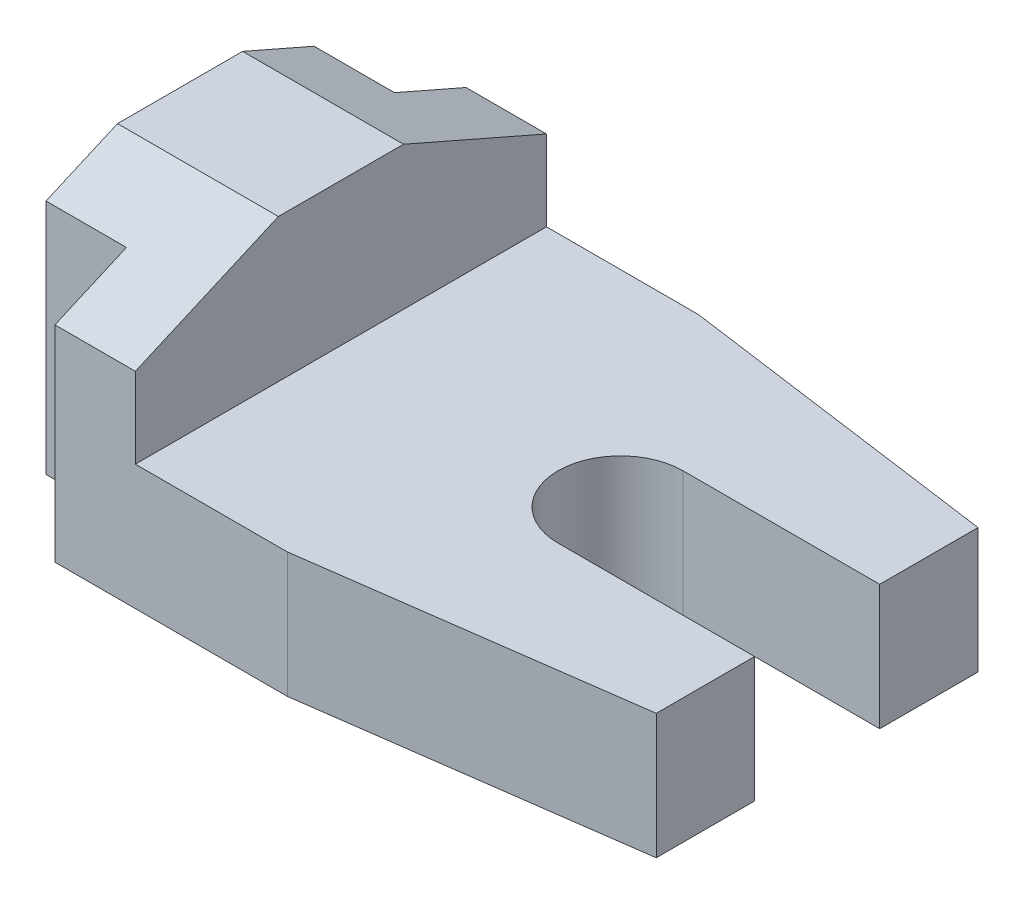
ISO-10303-21;
HEADER;
FILE_DESCRIPTION(('STEP AP214'),'2;1');
FILE_NAME('part.step','',(''),(''),'','','');
FILE_SCHEMA(('AUTOMOTIVE_DESIGN { 1 0 10303 214 1 1 1 1 }'));
ENDSEC;
DATA;
#1=APPLICATION_CONTEXT('core data for automotive mechanical design processes');
#2=APPLICATION_PROTOCOL_DEFINITION('international standard','automotive_design',2000,#1);
#3=PRODUCT_CONTEXT('',#1,'mechanical');
#4=PRODUCT('Part','Part','',(#3));
#5=PRODUCT_RELATED_PRODUCT_CATEGORY('part','',(#4));
#6=PRODUCT_DEFINITION_FORMATION('','',#4);
#7=PRODUCT_DEFINITION_CONTEXT('part definition',#1,'design');
#8=PRODUCT_DEFINITION('design','',#6,#7);
#9=PRODUCT_DEFINITION_SHAPE('','',#8);
#10=(LENGTH_UNIT() NAMED_UNIT(*) SI_UNIT(.MILLI.,.METRE.));
#11=(NAMED_UNIT(*) PLANE_ANGLE_UNIT() SI_UNIT($,.RADIAN.));
#12=(NAMED_UNIT(*) SI_UNIT($,.STERADIAN.) SOLID_ANGLE_UNIT());
#13=UNCERTAINTY_MEASURE_WITH_UNIT(LENGTH_MEASURE(1.E-05),#10,'distance_accuracy_value','');
#14=(GEOMETRIC_REPRESENTATION_CONTEXT(3) GLOBAL_UNCERTAINTY_ASSIGNED_CONTEXT((#13)) GLOBAL_UNIT_ASSIGNED_CONTEXT((#10,
#11,#12)) REPRESENTATION_CONTEXT('',''));
#15=CARTESIAN_POINT('',(0.,0.,0.));
#16=DIRECTION('',(0.,0.,1.));
#17=DIRECTION('',(1.,0.,0.));
#18=AXIS2_PLACEMENT_3D('',#15,#16,#17);
#19=CARTESIAN_POINT('',(40.2808988764045,7.,0.));
#20=DIRECTION('',(0.,1.,0.));
#21=DIRECTION('',(0.,0.,1.));
#22=AXIS2_PLACEMENT_3D('',#19,#20,#21);
#23=PLANE('',#22);
#24=DIRECTION('',(-1.,0.,0.));
#25=VECTOR('',#24,1.);
#26=CARTESIAN_POINT('',(0.,7.,-23.));
#27=LINE('',#26,#25);
#28=CARTESIAN_POINT('',(26.,7.,-23.));
#29=VERTEX_POINT('',#28);
#30=CARTESIAN_POINT('',(9.,7.,-23.));
#31=VERTEX_POINT('',#30);
#32=EDGE_CURVE('E254',#29,#31,#27,.T.);
#33=ORIENTED_EDGE('',*,*,#32,.T.);
#34=DIRECTION('',(0.,0.,1.));
#35=VECTOR('',#34,1.);
#36=CARTESIAN_POINT('',(9.,7.,0.));
#37=LINE('',#36,#35);
#38=CARTESIAN_POINT('',(9.,7.,23.));
#39=VERTEX_POINT('',#38);
#40=EDGE_CURVE('E233',#31,#39,#37,.T.);
#41=ORIENTED_EDGE('',*,*,#40,.T.);
#42=DIRECTION('',(1.,0.,0.));
#43=VECTOR('',#42,1.);
#44=CARTESIAN_POINT('',(0.,7.,23.));
#45=LINE('',#44,#43);
#46=CARTESIAN_POINT('',(26.,7.,23.));
#47=VERTEX_POINT('',#46);
#48=EDGE_CURVE('E236',#39,#47,#45,.T.);
#49=ORIENTED_EDGE('',*,*,#48,.T.);
#50=DIRECTION('',(0.990636874029976,0.,-0.136523198805618));
#51=VECTOR('',#50,1.);
#52=CARTESIAN_POINT('',(26.,7.,23.));
#53=LINE('',#52,#51);
#54=CARTESIAN_POINT('',(62.2808988764045,7.,18.));
#55=VERTEX_POINT('',#54);
#56=EDGE_CURVE('E238',#47,#55,#53,.T.);
#57=ORIENTED_EDGE('',*,*,#56,.T.);
#58=DIRECTION('',(0.,0.,-1.));
#59=VECTOR('',#58,1.);
#60=CARTESIAN_POINT('',(62.2808988764045,7.,7.));
#61=LINE('',#60,#59);
#62=CARTESIAN_POINT('',(62.2808988764045,7.,7.));
#63=VERTEX_POINT('',#62);
#64=EDGE_CURVE('E244',#55,#63,#61,.T.);
#65=ORIENTED_EDGE('',*,*,#64,.T.);
#66=DIRECTION('',(-1.,0.,0.));
#67=VECTOR('',#66,1.);
#68=CARTESIAN_POINT('',(40.2808988764045,7.,7.));
#69=LINE('',#68,#67);
#70=CARTESIAN_POINT('',(40.2808988764045,7.,7.));
#71=VERTEX_POINT('',#70);
#72=EDGE_CURVE('E245',#63,#71,#69,.T.);
#73=ORIENTED_EDGE('',*,*,#72,.T.);
#74=CARTESIAN_POINT('',(40.2808988764045,7.,0.));
#75=DIRECTION('',(0.,-1.,0.));
#76=DIRECTION('',(0.,0.,1.));
#77=AXIS2_PLACEMENT_3D('',#74,#75,#76);
#78=CIRCLE('',#77,7.);
#79=CARTESIAN_POINT('',(40.2808988764045,7.,-7.));
#80=VERTEX_POINT('',#79);
#81=EDGE_CURVE('E246',#71,#80,#78,.T.);
#82=ORIENTED_EDGE('',*,*,#81,.T.);
#83=DIRECTION('',(1.,0.,0.));
#84=VECTOR('',#83,1.);
#85=CARTESIAN_POINT('',(40.2808988764045,7.,-7.));
#86=LINE('',#85,#84);
#87=CARTESIAN_POINT('',(62.2808988764045,7.,-7.));
#88=VERTEX_POINT('',#87);
#89=EDGE_CURVE('E248',#80,#88,#86,.T.);
#90=ORIENTED_EDGE('',*,*,#89,.T.);
#91=DIRECTION('',(0.,0.,-1.));
#92=VECTOR('',#91,1.);
#93=CARTESIAN_POINT('',(62.2808988764045,7.,-7.));
#94=LINE('',#93,#92);
#95=CARTESIAN_POINT('',(62.2808988764045,7.,-18.));
#96=VERTEX_POINT('',#95);
#97=EDGE_CURVE('E253',#88,#96,#94,.T.);
#98=ORIENTED_EDGE('',*,*,#97,.T.);
#99=DIRECTION('',(-0.990636874029975,0.,-0.136523198805618));
#100=VECTOR('',#99,1.);
#101=CARTESIAN_POINT('',(26.,7.,-23.));
#102=LINE('',#101,#100);
#103=EDGE_CURVE('E251',#96,#29,#102,.T.);
#104=ORIENTED_EDGE('',*,*,#103,.T.);
#105=EDGE_LOOP('',(#33,#41,#49,#57,#65,#73,#82,#90,#98,#104));
#106=FACE_BOUND('',#105,.T.);
#107=ADVANCED_FACE('F39',(#106),#23,.T.);
#108=CARTESIAN_POINT('',(0.,7.,23.));
#109=DIRECTION('',(0.,0.,-1.));
#110=DIRECTION('',(-1.,0.,0.));
#111=AXIS2_PLACEMENT_3D('',#108,#109,#110);
#112=PLANE('',#111);
#113=DIRECTION('',(1.,0.,0.));
#114=VECTOR('',#113,1.);
#115=CARTESIAN_POINT('',(-9.,16.,23.));
#116=LINE('',#115,#114);
#117=CARTESIAN_POINT('',(0.,16.,23.));
#118=VERTEX_POINT('',#117);
#119=CARTESIAN_POINT('',(9.,16.,23.));
#120=VERTEX_POINT('',#119);
#121=EDGE_CURVE('E231',#118,#120,#116,.T.);
#122=ORIENTED_EDGE('',*,*,#121,.F.);
#123=DIRECTION('',(0.,1.,0.));
#124=VECTOR('',#123,1.);
#125=CARTESIAN_POINT('',(0.,-7.,23.));
#126=LINE('',#125,#124);
#127=CARTESIAN_POINT('',(0.,-7.,23.));
#128=VERTEX_POINT('',#127);
#129=EDGE_CURVE('E193',#128,#118,#126,.T.);
#130=ORIENTED_EDGE('',*,*,#129,.F.);
#131=DIRECTION('',(1.,0.,0.));
#132=VECTOR('',#131,1.);
#133=CARTESIAN_POINT('',(0.,-7.,23.));
#134=LINE('',#133,#132);
#135=CARTESIAN_POINT('',(26.,-7.,23.));
#136=VERTEX_POINT('',#135);
#137=EDGE_CURVE('E240',#128,#136,#134,.T.);
#138=ORIENTED_EDGE('',*,*,#137,.T.);
#139=DIRECTION('',(0.,-1.,0.));
#140=VECTOR('',#139,1.);
#141=CARTESIAN_POINT('',(26.,7.,23.));
#142=LINE('',#141,#140);
#143=EDGE_CURVE('E293',#47,#136,#142,.T.);
#144=ORIENTED_EDGE('',*,*,#143,.F.);
#145=ORIENTED_EDGE('',*,*,#48,.F.);
#146=DIRECTION('',(0.,1.,0.));
#147=VECTOR('',#146,1.);
#148=CARTESIAN_POINT('',(9.,7.,23.));
#149=LINE('',#148,#147);
#150=EDGE_CURVE('E201',#39,#120,#149,.T.);
#151=ORIENTED_EDGE('',*,*,#150,.T.);
#152=EDGE_LOOP('',(#122,#130,#138,#144,#145,#151));
#153=FACE_BOUND('',#152,.T.);
#154=ADVANCED_FACE('F41',(#153),#112,.F.);
#155=CARTESIAN_POINT('',(26.,7.,23.));
#156=DIRECTION('',(-0.136523198805618,0.,-0.990636874029976));
#157=DIRECTION('',(-0.990636874029976,0.,0.136523198805618));
#158=AXIS2_PLACEMENT_3D('',#155,#156,#157);
#159=PLANE('',#158);
#160=DIRECTION('',(0.990636874029976,0.,-0.136523198805618));
#161=VECTOR('',#160,1.);
#162=CARTESIAN_POINT('',(26.,-7.,23.));
#163=LINE('',#162,#161);
#164=CARTESIAN_POINT('',(62.2808988764045,-7.,18.));
#165=VERTEX_POINT('',#164);
#166=EDGE_CURVE('E257',#136,#165,#163,.T.);
#167=ORIENTED_EDGE('',*,*,#166,.T.);
#168=DIRECTION('',(0.,-1.,0.));
#169=VECTOR('',#168,1.);
#170=CARTESIAN_POINT('',(62.2808988764045,7.,18.));
#171=LINE('',#170,#169);
#172=EDGE_CURVE('E295',#55,#165,#171,.T.);
#173=ORIENTED_EDGE('',*,*,#172,.F.);
#174=ORIENTED_EDGE('',*,*,#56,.F.);
#175=ORIENTED_EDGE('',*,*,#143,.T.);
#176=EDGE_LOOP('',(#167,#173,#174,#175));
#177=FACE_BOUND('',#176,.T.);
#178=ADVANCED_FACE('F340',(#177),#159,.F.);
#179=CARTESIAN_POINT('',(62.2808988764045,7.,7.));
#180=DIRECTION('',(-1.,0.,0.));
#181=DIRECTION('',(0.,0.,1.));
#182=AXIS2_PLACEMENT_3D('',#179,#180,#181);
#183=PLANE('',#182);
#184=DIRECTION('',(0.,0.,-1.));
#185=VECTOR('',#184,1.);
#186=CARTESIAN_POINT('',(62.2808988764045,-7.,7.));
#187=LINE('',#186,#185);
#188=CARTESIAN_POINT('',(62.2808988764045,-7.,7.));
#189=VERTEX_POINT('',#188);
#190=EDGE_CURVE('E265',#165,#189,#187,.T.);
#191=ORIENTED_EDGE('',*,*,#190,.T.);
#192=DIRECTION('',(0.,-1.,0.));
#193=VECTOR('',#192,1.);
#194=CARTESIAN_POINT('',(62.2808988764045,7.,7.));
#195=LINE('',#194,#193);
#196=EDGE_CURVE('E288',#63,#189,#195,.T.);
#197=ORIENTED_EDGE('',*,*,#196,.F.);
#198=ORIENTED_EDGE('',*,*,#64,.F.);
#199=ORIENTED_EDGE('',*,*,#172,.T.);
#200=EDGE_LOOP('',(#191,#197,#198,#199));
#201=FACE_BOUND('',#200,.T.);
#202=ADVANCED_FACE('F334',(#201),#183,.F.);
#203=CARTESIAN_POINT('',(40.2808988764045,7.,7.));
#204=DIRECTION('',(0.,0.,1.));
#205=DIRECTION('',(1.,0.,0.));
#206=AXIS2_PLACEMENT_3D('',#203,#204,#205);
#207=PLANE('',#206);
#208=DIRECTION('',(-1.,0.,0.));
#209=VECTOR('',#208,1.);
#210=CARTESIAN_POINT('',(40.2808988764045,-7.,7.));
#211=LINE('',#210,#209);
#212=CARTESIAN_POINT('',(40.2808988764045,-7.,7.));
#213=VERTEX_POINT('',#212);
#214=EDGE_CURVE('E262',#189,#213,#211,.T.);
#215=ORIENTED_EDGE('',*,*,#214,.T.);
#216=DIRECTION('',(0.,-1.,0.));
#217=VECTOR('',#216,1.);
#218=CARTESIAN_POINT('',(40.2808988764045,7.,7.));
#219=LINE('',#218,#217);
#220=EDGE_CURVE('E289',#71,#213,#219,.T.);
#221=ORIENTED_EDGE('',*,*,#220,.F.);
#222=ORIENTED_EDGE('',*,*,#72,.F.);
#223=ORIENTED_EDGE('',*,*,#196,.T.);
#224=EDGE_LOOP('',(#215,#221,#222,#223));
#225=FACE_BOUND('',#224,.T.);
#226=ADVANCED_FACE('F328',(#225),#207,.F.);
#227=CARTESIAN_POINT('',(40.2808988764045,7.,0.));
#228=DIRECTION('',(0.,-1.,0.));
#229=DIRECTION('',(0.,0.,-1.));
#230=AXIS2_PLACEMENT_3D('',#227,#228,#229);
#231=CYLINDRICAL_SURFACE('',#230,7.);
#232=CARTESIAN_POINT('',(40.2808988764045,-7.,0.));
#233=DIRECTION('',(0.,-1.,0.));
#234=DIRECTION('',(0.,0.,1.));
#235=AXIS2_PLACEMENT_3D('',#232,#233,#234);
#236=CIRCLE('',#235,7.);
#237=CARTESIAN_POINT('',(40.2808988764045,-7.,-7.));
#238=VERTEX_POINT('',#237);
#239=EDGE_CURVE('E266',#213,#238,#236,.T.);
#240=ORIENTED_EDGE('',*,*,#239,.T.);
#241=DIRECTION('',(0.,-1.,0.));
#242=VECTOR('',#241,1.);
#243=CARTESIAN_POINT('',(40.2808988764045,7.,-7.));
#244=LINE('',#243,#242);
#245=EDGE_CURVE('E284',#80,#238,#244,.T.);
#246=ORIENTED_EDGE('',*,*,#245,.F.);
#247=ORIENTED_EDGE('',*,*,#81,.F.);
#248=ORIENTED_EDGE('',*,*,#220,.T.);
#249=EDGE_LOOP('',(#240,#246,#247,#248));
#250=FACE_BOUND('',#249,.T.);
#251=ADVANCED_FACE('F322',(#250),#231,.F.);
#252=CARTESIAN_POINT('',(40.2808988764045,7.,-7.));
#253=DIRECTION('',(0.,0.,-1.));
#254=DIRECTION('',(-1.,0.,0.));
#255=AXIS2_PLACEMENT_3D('',#252,#253,#254);
#256=PLANE('',#255);
#257=DIRECTION('',(1.,0.,0.));
#258=VECTOR('',#257,1.);
#259=CARTESIAN_POINT('',(40.2808988764045,-7.,-7.));
#260=LINE('',#259,#258);
#261=CARTESIAN_POINT('',(62.2808988764045,-7.,-7.));
#262=VERTEX_POINT('',#261);
#263=EDGE_CURVE('E268',#238,#262,#260,.T.);
#264=ORIENTED_EDGE('',*,*,#263,.T.);
#265=DIRECTION('',(0.,-1.,0.));
#266=VECTOR('',#265,1.);
#267=CARTESIAN_POINT('',(62.2808988764045,7.,-7.));
#268=LINE('',#267,#266);
#269=EDGE_CURVE('E278',#88,#262,#268,.T.);
#270=ORIENTED_EDGE('',*,*,#269,.F.);
#271=ORIENTED_EDGE('',*,*,#89,.F.);
#272=ORIENTED_EDGE('',*,*,#245,.T.);
#273=EDGE_LOOP('',(#264,#270,#271,#272));
#274=FACE_BOUND('',#273,.T.);
#275=ADVANCED_FACE('F318',(#274),#256,.F.);
#276=CARTESIAN_POINT('',(62.2808988764045,7.,-7.));
#277=DIRECTION('',(-1.,0.,0.));
#278=DIRECTION('',(0.,0.,1.));
#279=AXIS2_PLACEMENT_3D('',#276,#277,#278);
#280=PLANE('',#279);
#281=DIRECTION('',(0.,0.,-1.));
#282=VECTOR('',#281,1.);
#283=CARTESIAN_POINT('',(62.2808988764045,-7.,-7.));
#284=LINE('',#283,#282);
#285=CARTESIAN_POINT('',(62.2808988764045,-7.,-18.));
#286=VERTEX_POINT('',#285);
#287=EDGE_CURVE('E269',#262,#286,#284,.T.);
#288=ORIENTED_EDGE('',*,*,#287,.T.);
#289=DIRECTION('',(0.,-1.,0.));
#290=VECTOR('',#289,1.);
#291=CARTESIAN_POINT('',(62.2808988764045,7.,-18.));
#292=LINE('',#291,#290);
#293=EDGE_CURVE('E280',#96,#286,#292,.T.);
#294=ORIENTED_EDGE('',*,*,#293,.F.);
#295=ORIENTED_EDGE('',*,*,#97,.F.);
#296=ORIENTED_EDGE('',*,*,#269,.T.);
#297=EDGE_LOOP('',(#288,#294,#295,#296));
#298=FACE_BOUND('',#297,.T.);
#299=ADVANCED_FACE('F314',(#298),#280,.F.);
#300=CARTESIAN_POINT('',(26.,7.,-23.));
#301=DIRECTION('',(-0.136523198805618,0.,0.990636874029975));
#302=DIRECTION('',(0.990636874029976,0.,0.136523198805618));
#303=AXIS2_PLACEMENT_3D('',#300,#301,#302);
#304=PLANE('',#303);
#305=DIRECTION('',(-0.990636874029975,0.,-0.136523198805618));
#306=VECTOR('',#305,1.);
#307=CARTESIAN_POINT('',(26.,-7.,-23.));
#308=LINE('',#307,#306);
#309=CARTESIAN_POINT('',(26.,-7.,-23.));
#310=VERTEX_POINT('',#309);
#311=EDGE_CURVE('E275',#286,#310,#308,.T.);
#312=ORIENTED_EDGE('',*,*,#311,.T.);
#313=DIRECTION('',(0.,-1.,0.));
#314=VECTOR('',#313,1.);
#315=CARTESIAN_POINT('',(26.,7.,-23.));
#316=LINE('',#315,#314);
#317=EDGE_CURVE('E256',#29,#310,#316,.T.);
#318=ORIENTED_EDGE('',*,*,#317,.F.);
#319=ORIENTED_EDGE('',*,*,#103,.F.);
#320=ORIENTED_EDGE('',*,*,#293,.T.);
#321=EDGE_LOOP('',(#312,#318,#319,#320));
#322=FACE_BOUND('',#321,.T.);
#323=ADVANCED_FACE('F310',(#322),#304,.F.);
#324=CARTESIAN_POINT('',(0.,7.,-23.));
#325=DIRECTION('',(0.,0.,1.));
#326=DIRECTION('',(1.,0.,0.));
#327=AXIS2_PLACEMENT_3D('',#324,#325,#326);
#328=PLANE('',#327);
#329=DIRECTION('',(-1.,0.,0.));
#330=VECTOR('',#329,1.);
#331=CARTESIAN_POINT('',(0.,-7.,-23.));
#332=LINE('',#331,#330);
#333=CARTESIAN_POINT('',(0.,-7.00000000000001,-23.));
#334=VERTEX_POINT('',#333);
#335=EDGE_CURVE('E241',#310,#334,#332,.T.);
#336=ORIENTED_EDGE('',*,*,#335,.T.);
#337=DIRECTION('',(0.,1.,0.));
#338=VECTOR('',#337,1.);
#339=CARTESIAN_POINT('',(0.,-7.00000000000001,-23.));
#340=LINE('',#339,#338);
#341=CARTESIAN_POINT('',(0.,16.,-23.));
#342=VERTEX_POINT('',#341);
#343=EDGE_CURVE('E168',#334,#342,#340,.T.);
#344=ORIENTED_EDGE('',*,*,#343,.T.);
#345=DIRECTION('',(1.,0.,0.));
#346=VECTOR('',#345,1.);
#347=CARTESIAN_POINT('',(-9.,16.,-23.));
#348=LINE('',#347,#346);
#349=CARTESIAN_POINT('',(9.,16.,-23.));
#350=VERTEX_POINT('',#349);
#351=EDGE_CURVE('E213',#342,#350,#348,.T.);
#352=ORIENTED_EDGE('',*,*,#351,.T.);
#353=DIRECTION('',(0.,-1.,0.));
#354=VECTOR('',#353,1.);
#355=CARTESIAN_POINT('',(9.,7.,-23.));
#356=LINE('',#355,#354);
#357=EDGE_CURVE('E206',#350,#31,#356,.T.);
#358=ORIENTED_EDGE('',*,*,#357,.T.);
#359=ORIENTED_EDGE('',*,*,#32,.F.);
#360=ORIENTED_EDGE('',*,*,#317,.T.);
#361=EDGE_LOOP('',(#336,#344,#352,#358,#359,#360));
#362=FACE_BOUND('',#361,.T.);
#363=ADVANCED_FACE('F301',(#362),#328,.F.);
#364=CARTESIAN_POINT('',(40.2808988764045,-7.,0.));
#365=DIRECTION('',(0.,1.,0.));
#366=DIRECTION('',(0.,0.,1.));
#367=AXIS2_PLACEMENT_3D('',#364,#365,#366);
#368=PLANE('',#367);
#369=DIRECTION('',(1.,0.,0.));
#370=VECTOR('',#369,1.);
#371=CARTESIAN_POINT('',(-9.00000000000001,-7.00000000000001,-15.));
#372=LINE('',#371,#370);
#373=CARTESIAN_POINT('',(-9.,-7.,-15.));
#374=VERTEX_POINT('',#373);
#375=CARTESIAN_POINT('',(0.,-7.00000000000001,-15.));
#376=VERTEX_POINT('',#375);
#377=EDGE_CURVE('E62',#374,#376,#372,.T.);
#378=ORIENTED_EDGE('',*,*,#377,.T.);
#379=DIRECTION('',(0.,0.,-1.));
#380=VECTOR('',#379,1.);
#381=CARTESIAN_POINT('',(0.,-7.00000000000001,-15.));
#382=LINE('',#381,#380);
#383=EDGE_CURVE('E173',#376,#334,#382,.T.);
#384=ORIENTED_EDGE('',*,*,#383,.T.);
#385=ORIENTED_EDGE('',*,*,#335,.F.);
#386=ORIENTED_EDGE('',*,*,#311,.F.);
#387=ORIENTED_EDGE('',*,*,#287,.F.);
#388=ORIENTED_EDGE('',*,*,#263,.F.);
#389=ORIENTED_EDGE('',*,*,#239,.F.);
#390=ORIENTED_EDGE('',*,*,#214,.F.);
#391=ORIENTED_EDGE('',*,*,#190,.F.);
#392=ORIENTED_EDGE('',*,*,#166,.F.);
#393=ORIENTED_EDGE('',*,*,#137,.F.);
#394=DIRECTION('',(0.,0.,-1.));
#395=VECTOR('',#394,1.);
#396=CARTESIAN_POINT('',(0.,-7.,15.));
#397=LINE('',#396,#395);
#398=CARTESIAN_POINT('',(0.,-7.,15.));
#399=VERTEX_POINT('',#398);
#400=EDGE_CURVE('E186',#128,#399,#397,.T.);
#401=ORIENTED_EDGE('',*,*,#400,.T.);
#402=DIRECTION('',(-1.,0.,0.));
#403=VECTOR('',#402,1.);
#404=CARTESIAN_POINT('',(-8.99999999999999,-7.,15.));
#405=LINE('',#404,#403);
#406=CARTESIAN_POINT('',(-8.99999999999999,-7.,15.));
#407=VERTEX_POINT('',#406);
#408=EDGE_CURVE('E188',#399,#407,#405,.T.);
#409=ORIENTED_EDGE('',*,*,#408,.T.);
#410=DIRECTION('',(0.,0.,1.));
#411=VECTOR('',#410,1.);
#412=CARTESIAN_POINT('',(-9.,-7.,-23.));
#413=LINE('',#412,#411);
#414=EDGE_CURVE('E183',#374,#407,#413,.T.);
#415=ORIENTED_EDGE('',*,*,#414,.F.);
#416=EDGE_LOOP('',(#378,#384,#385,#386,#387,#388,#389,#390,#391,#392,#393,#401,#409,#415));
#417=FACE_BOUND('',#416,.T.);
#418=ADVANCED_FACE('F185',(#417),#368,.F.);
#419=CARTESIAN_POINT('',(-9.,23.,7.));
#420=DIRECTION('',(0.,-0.916157334902189,-0.400818834019708));
#421=DIRECTION('',(0.,0.400818834019708,-0.916157334902189));
#422=AXIS2_PLACEMENT_3D('',#419,#420,#421);
#423=PLANE('',#422);
#424=DIRECTION('',(0.,0.400818834019708,-0.916157334902189));
#425=VECTOR('',#424,1.);
#426=CARTESIAN_POINT('',(-9.,23.,7.));
#427=LINE('',#426,#425);
#428=CARTESIAN_POINT('',(-9.,19.5,15.));
#429=VERTEX_POINT('',#428);
#430=CARTESIAN_POINT('',(-9.,23.,7.));
#431=VERTEX_POINT('',#430);
#432=EDGE_CURVE('E202',#429,#431,#427,.T.);
#433=ORIENTED_EDGE('',*,*,#432,.F.);
#434=DIRECTION('',(1.,0.,0.));
#435=VECTOR('',#434,1.);
#436=CARTESIAN_POINT('',(-8.99999999999999,19.5,15.));
#437=LINE('',#436,#435);
#438=CARTESIAN_POINT('',(0.,19.5,15.));
#439=VERTEX_POINT('',#438);
#440=EDGE_CURVE('E53',#429,#439,#437,.T.);
#441=ORIENTED_EDGE('',*,*,#440,.T.);
#442=DIRECTION('',(0.,-0.400818834019708,0.916157334902189));
#443=VECTOR('',#442,1.);
#444=CARTESIAN_POINT('',(0.,23.,6.99999999999999));
#445=LINE('',#444,#443);
#446=EDGE_CURVE('E11',#439,#118,#445,.T.);
#447=ORIENTED_EDGE('',*,*,#446,.T.);
#448=ORIENTED_EDGE('',*,*,#121,.T.);
#449=DIRECTION('',(0.,0.400818834019708,-0.916157334902189));
#450=VECTOR('',#449,1.);
#451=CARTESIAN_POINT('',(9.,23.,7.));
#452=LINE('',#451,#450);
#453=CARTESIAN_POINT('',(9.,23.,7.));
#454=VERTEX_POINT('',#453);
#455=EDGE_CURVE('E216',#120,#454,#452,.T.);
#456=ORIENTED_EDGE('',*,*,#455,.T.);
#457=DIRECTION('',(1.,0.,0.));
#458=VECTOR('',#457,1.);
#459=CARTESIAN_POINT('',(-9.,23.,7.));
#460=LINE('',#459,#458);
#461=EDGE_CURVE('E228',#431,#454,#460,.T.);
#462=ORIENTED_EDGE('',*,*,#461,.F.);
#463=EDGE_LOOP('',(#433,#441,#447,#448,#456,#462));
#464=FACE_BOUND('',#463,.T.);
#465=ADVANCED_FACE('F349',(#464),#423,.F.);
#466=CARTESIAN_POINT('',(-9.,23.,-7.));
#467=DIRECTION('',(0.,-1.,0.));
#468=DIRECTION('',(0.,0.,-1.));
#469=AXIS2_PLACEMENT_3D('',#466,#467,#468);
#470=PLANE('',#469);
#471=DIRECTION('',(0.,0.,-1.));
#472=VECTOR('',#471,1.);
#473=CARTESIAN_POINT('',(9.,23.,-7.));
#474=LINE('',#473,#472);
#475=CARTESIAN_POINT('',(9.,23.,-7.));
#476=VERTEX_POINT('',#475);
#477=EDGE_CURVE('E217',#454,#476,#474,.T.);
#478=ORIENTED_EDGE('',*,*,#477,.T.);
#479=DIRECTION('',(1.,0.,0.));
#480=VECTOR('',#479,1.);
#481=CARTESIAN_POINT('',(-9.,23.,-7.));
#482=LINE('',#481,#480);
#483=CARTESIAN_POINT('',(-9.,23.,-7.));
#484=VERTEX_POINT('',#483);
#485=EDGE_CURVE('E226',#484,#476,#482,.T.);
#486=ORIENTED_EDGE('',*,*,#485,.F.);
#487=DIRECTION('',(0.,0.,-1.));
#488=VECTOR('',#487,1.);
#489=CARTESIAN_POINT('',(-9.,23.,-7.));
#490=LINE('',#489,#488);
#491=EDGE_CURVE('E208',#431,#484,#490,.T.);
#492=ORIENTED_EDGE('',*,*,#491,.F.);
#493=ORIENTED_EDGE('',*,*,#461,.T.);
#494=EDGE_LOOP('',(#478,#486,#492,#493));
#495=FACE_BOUND('',#494,.T.);
#496=ADVANCED_FACE('F471',(#495),#470,.F.);
#497=CARTESIAN_POINT('',(-9.,16.,-23.));
#498=DIRECTION('',(0.,-0.916157334902189,0.400818834019708));
#499=DIRECTION('',(0.,-0.400818834019708,-0.916157334902189));
#500=AXIS2_PLACEMENT_3D('',#497,#498,#499);
#501=PLANE('',#500);
#502=ORIENTED_EDGE('',*,*,#351,.F.);
#503=DIRECTION('',(0.,0.400818834019708,0.916157334902189));
#504=VECTOR('',#503,1.);
#505=CARTESIAN_POINT('',(0.,16.,-23.));
#506=LINE('',#505,#504);
#507=CARTESIAN_POINT('',(0.,19.5,-15.));
#508=VERTEX_POINT('',#507);
#509=EDGE_CURVE('E50',#342,#508,#506,.T.);
#510=ORIENTED_EDGE('',*,*,#509,.T.);
#511=DIRECTION('',(-1.,0.,0.));
#512=VECTOR('',#511,1.);
#513=CARTESIAN_POINT('',(-9.,19.5,-15.));
#514=LINE('',#513,#512);
#515=CARTESIAN_POINT('',(-9.00000000000001,19.5,-15.));
#516=VERTEX_POINT('',#515);
#517=EDGE_CURVE('E170',#508,#516,#514,.T.);
#518=ORIENTED_EDGE('',*,*,#517,.T.);
#519=DIRECTION('',(0.,-0.400818834019708,-0.916157334902189));
#520=VECTOR('',#519,1.);
#521=CARTESIAN_POINT('',(-9.,16.,-23.));
#522=LINE('',#521,#520);
#523=EDGE_CURVE('E209',#484,#516,#522,.T.);
#524=ORIENTED_EDGE('',*,*,#523,.F.);
#525=ORIENTED_EDGE('',*,*,#485,.T.);
#526=DIRECTION('',(0.,-0.400818834019708,-0.916157334902189));
#527=VECTOR('',#526,1.);
#528=CARTESIAN_POINT('',(9.,16.,-23.));
#529=LINE('',#528,#527);
#530=EDGE_CURVE('E219',#476,#350,#529,.T.);
#531=ORIENTED_EDGE('',*,*,#530,.T.);
#532=EDGE_LOOP('',(#502,#510,#518,#524,#525,#531));
#533=FACE_BOUND('',#532,.T.);
#534=ADVANCED_FACE('F298',(#533),#501,.F.);
#535=CARTESIAN_POINT('',(-9.,0.,0.));
#536=DIRECTION('',(-1.,0.,0.));
#537=DIRECTION('',(0.,0.,1.));
#538=AXIS2_PLACEMENT_3D('',#535,#536,#537);
#539=PLANE('',#538);
#540=DIRECTION('',(0.,1.,0.));
#541=VECTOR('',#540,1.);
#542=CARTESIAN_POINT('',(-9.00000000000001,-7.00000000000001,-15.));
#543=LINE('',#542,#541);
#544=EDGE_CURVE('E171',#374,#516,#543,.T.);
#545=ORIENTED_EDGE('',*,*,#544,.F.);
#546=ORIENTED_EDGE('',*,*,#414,.T.);
#547=DIRECTION('',(0.,1.,0.));
#548=VECTOR('',#547,1.);
#549=CARTESIAN_POINT('',(-8.99999999999999,-7.,15.));
#550=LINE('',#549,#548);
#551=EDGE_CURVE('E196',#407,#429,#550,.T.);
#552=ORIENTED_EDGE('',*,*,#551,.T.);
#553=ORIENTED_EDGE('',*,*,#432,.T.);
#554=ORIENTED_EDGE('',*,*,#491,.T.);
#555=ORIENTED_EDGE('',*,*,#523,.T.);
#556=EDGE_LOOP('',(#545,#546,#552,#553,#554,#555));
#557=FACE_BOUND('',#556,.T.);
#558=ADVANCED_FACE('F354',(#557),#539,.T.);
#559=CARTESIAN_POINT('',(9.,0.,0.));
#560=DIRECTION('',(-1.,0.,0.));
#561=DIRECTION('',(0.,0.,1.));
#562=AXIS2_PLACEMENT_3D('',#559,#560,#561);
#563=PLANE('',#562);
#564=ORIENTED_EDGE('',*,*,#40,.F.);
#565=ORIENTED_EDGE('',*,*,#357,.F.);
#566=ORIENTED_EDGE('',*,*,#530,.F.);
#567=ORIENTED_EDGE('',*,*,#477,.F.);
#568=ORIENTED_EDGE('',*,*,#455,.F.);
#569=ORIENTED_EDGE('',*,*,#150,.F.);
#570=EDGE_LOOP('',(#564,#565,#566,#567,#568,#569));
#571=FACE_BOUND('',#570,.T.);
#572=ADVANCED_FACE('F365',(#571),#563,.F.);
#573=CARTESIAN_POINT('',(0.,-7.,15.));
#574=DIRECTION('',(1.,0.,0.));
#575=DIRECTION('',(0.,0.,-1.));
#576=AXIS2_PLACEMENT_3D('',#573,#574,#575);
#577=PLANE('',#576);
#578=DIRECTION('',(0.,1.,0.));
#579=VECTOR('',#578,1.);
#580=CARTESIAN_POINT('',(0.,-7.,15.));
#581=LINE('',#580,#579);
#582=EDGE_CURVE('E198',#399,#439,#581,.T.);
#583=ORIENTED_EDGE('',*,*,#582,.F.);
#584=ORIENTED_EDGE('',*,*,#400,.F.);
#585=ORIENTED_EDGE('',*,*,#129,.T.);
#586=ORIENTED_EDGE('',*,*,#446,.F.);
#587=EDGE_LOOP('',(#583,#584,#585,#586));
#588=FACE_BOUND('',#587,.T.);
#589=ADVANCED_FACE('F347',(#588),#577,.F.);
#590=CARTESIAN_POINT('',(-8.99999999999999,-7.,15.));
#591=DIRECTION('',(0.,0.,-1.));
#592=DIRECTION('',(-1.,0.,0.));
#593=AXIS2_PLACEMENT_3D('',#590,#591,#592);
#594=PLANE('',#593);
#595=ORIENTED_EDGE('',*,*,#551,.F.);
#596=ORIENTED_EDGE('',*,*,#408,.F.);
#597=ORIENTED_EDGE('',*,*,#582,.T.);
#598=ORIENTED_EDGE('',*,*,#440,.F.);
#599=EDGE_LOOP('',(#595,#596,#597,#598));
#600=FACE_BOUND('',#599,.T.);
#601=ADVANCED_FACE('F359',(#600),#594,.F.);
#602=CARTESIAN_POINT('',(0.,-7.00000000000001,-15.));
#603=DIRECTION('',(1.,0.,0.));
#604=DIRECTION('',(0.,0.,-1.));
#605=AXIS2_PLACEMENT_3D('',#602,#603,#604);
#606=PLANE('',#605);
#607=ORIENTED_EDGE('',*,*,#343,.F.);
#608=ORIENTED_EDGE('',*,*,#383,.F.);
#609=DIRECTION('',(0.,1.,0.));
#610=VECTOR('',#609,1.);
#611=CARTESIAN_POINT('',(0.,-7.00000000000001,-15.));
#612=LINE('',#611,#610);
#613=EDGE_CURVE('E162',#376,#508,#612,.T.);
#614=ORIENTED_EDGE('',*,*,#613,.T.);
#615=ORIENTED_EDGE('',*,*,#509,.F.);
#616=EDGE_LOOP('',(#607,#608,#614,#615));
#617=FACE_BOUND('',#616,.T.);
#618=ADVANCED_FACE('F175',(#617),#606,.F.);
#619=CARTESIAN_POINT('',(-9.00000000000001,-7.00000000000001,-15.));
#620=DIRECTION('',(0.,0.,1.));
#621=DIRECTION('',(0.,-1.,0.));
#622=AXIS2_PLACEMENT_3D('',#619,#620,#621);
#623=PLANE('',#622);
#624=ORIENTED_EDGE('',*,*,#613,.F.);
#625=ORIENTED_EDGE('',*,*,#377,.F.);
#626=ORIENTED_EDGE('',*,*,#544,.T.);
#627=ORIENTED_EDGE('',*,*,#517,.F.);
#628=EDGE_LOOP('',(#624,#625,#626,#627));
#629=FACE_BOUND('',#628,.T.);
#630=ADVANCED_FACE('F164',(#629),#623,.F.);
#631=CLOSED_SHELL('',(#107,#154,#178,#202,#226,#251,#275,#299,#323,#363,#418,#465,#496,#534,
#558,#572,#589,#601,#618,#630));
#632=MANIFOLD_SOLID_BREP('B2',#631);
#633=ADVANCED_BREP_SHAPE_REPRESENTATION('',(#18,#632),#14);
#634=SHAPE_DEFINITION_REPRESENTATION(#9,#633);
ENDSEC;
END-ISO-10303-21;
